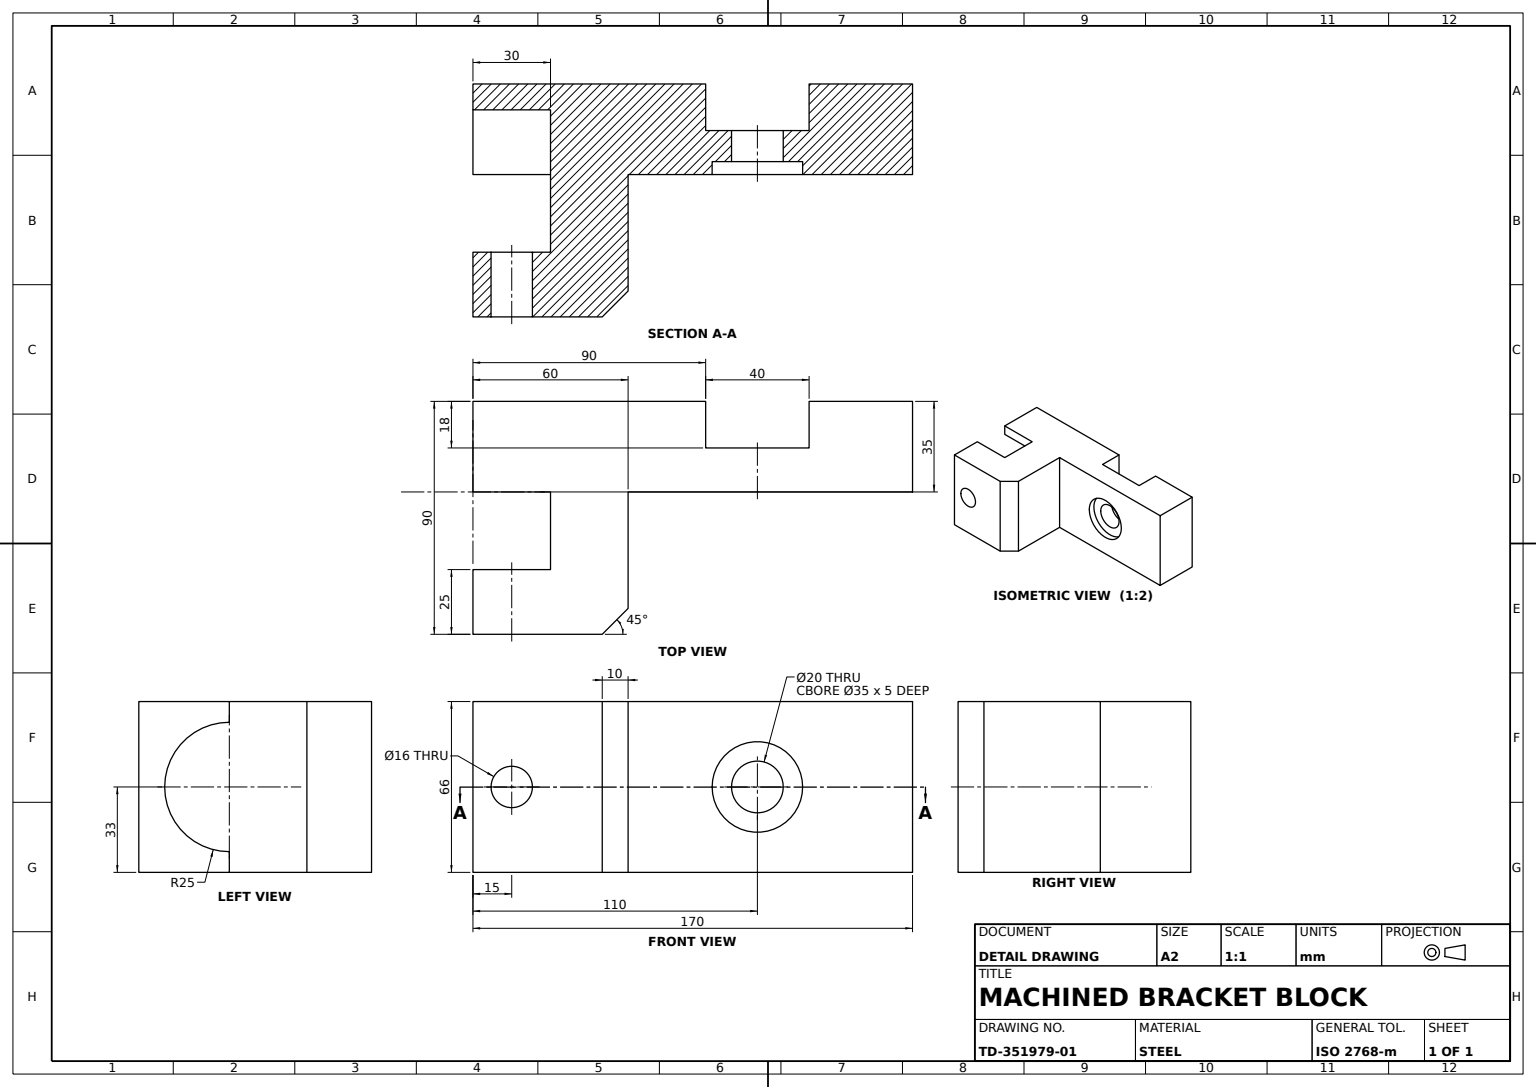
SolidWorks part; units mm, degrees
material "Plain Carbon Steel"
ref_plane "Front Plane" through (0, 0, 0) normal (0, 0, 1) x (1, 0, 0)
ref_plane "Top Plane" through (0, 0, 0) normal (0, 1, 0) x (1, 0, 0)
ref_plane "Right Plane" through (0, 0, 0) normal (1, 0, 0) x (0, 0, -1)
sketch "Base Block Profile" plane through (0, 0, 0) normal (0, 0, 1) x (1, 0, 0)
  line L0 (0, 0) -> (170, 0)
  line L1 (170, 0) -> (170, 66)
  line L2 (170, 66) -> (0, 66)
  line L3 (0, 66) -> (0, 0)
  dimension "D1" = 170
  dimension "D2" = 66
extrude "Base Block" add sketch "Base Block Profile" along normal blind 35
sketch "Slot Profile" plane through (0, 0, 0) normal (0, -1, 0) x (1, 0, 0)
  line L0 (170, 0) -> (110, 0)
  line L1 (0, 0) -> (170, 0) construction
  line L2 (170, 35) -> (170, 0) construction
  line L4 (110, 0) -> (130, 0)
  line L5 (130, 0) -> (90, 0)
  line L6 (130, 0) -> (130, 18)
  line L7 (130, 18) -> (90, 18)
  line L8 (90, 18) -> (90, 0)
  line M1 (0, 0) -> (170, 0)
  dimension "D1" = 40
  dimension "D2" = 60
  dimension "D3" = 18
extrude "Slot Cut" cut sketch "Slot Profile" against normal blind 66 contours L7 L8 L6 M1
sketch "Counterbore Ø35 Sketch" plane through (0, 0, 35) normal (0, 0, 1) x (1, 0, 0)
  line L0 (0, 66) -> (0, 0) construction
  line L1 (0, 0) -> (170, 0) construction
  circle A0 centre (110, 33) radius 17.5
  dimension "D1" = 35
  dimension "D2" = 35
  dimension "D3" = 110
  dimension "D4" = 33
extrude "Counterbore Ø35" cut sketch "Counterbore Ø35 Sketch" against normal blind 5
sketch "Hole Ø20 Sketch" plane through (0, 0, 30) normal (0, 0, 1) x (1, 0, 0)
  circle A0 centre (110, 33) radius 10
  dimension "D1" = 20
  dimension "D2" = 20
extrude "Hole Ø20" cut sketch "Hole Ø20 Sketch" against normal blind 12
sketch "Rounded Cut Sketch" plane through (0, 0, 0) normal (-1, 0, 0) x (0, 0, 1)
  line L0 (35, 66) -> (35, 0) construction
  line L1 (35, 58) -> (35, 8)
  arc A0 (35, 58) -> (35, 8) centre (35, 33) ccw
  dimension "D1" = 50
  dimension "D2" = 25
extrude "Rounded Cut" cut sketch "Rounded Cut Sketch" against normal blind 30
sketch "Side Lug Profile" plane through (0, 0, 0) normal (0, -1, 0) x (1, 0, 0)
  line L0 (170, 35) -> (170, 0) construction
  line L1 (0, 35) -> (170, 35) construction
  line L2 (30, 35) -> (30, 65)
  line L3 (30, 65) -> (0, 65)
  line L4 (0, 65) -> (0, 90)
  line L5 (0, 90) -> (50, 90)
  line L8 (60, 80) -> (60, 35)
  line L9 (60, 35) -> (30, 35)
  line L10 (50, 90) -> (60, 80)
  line L11 (30, 35) -> (60, 35)
  line L12 (130, 18) -> (90, 18) construction
  line M5 (170, 35) -> (0, 35)
  dimension "D1" = 110
  dimension "D2" = 120
  dimension "D3" = 62
  dimension "D4" = 72
extrude "Side Lug" add sketch "Side Lug Profile" against normal blind 66 contours L10 L5 L4 L3 L2 L8 M5
sketch "Lug Hole Ø16 Sketch" plane through (0, 0, 90) normal (0, 0, 1) x (1, 0, 0)
  line L0 (0, 66) -> (0, 0) construction
  line L2 (0, 0) -> (50, 0) construction
  circle A0 centre (15, 33) radius 8
  dimension "D1" = 16
  dimension "D3" = 16
  dimension "D2" = 15
  dimension "D4" = 33
extrude "Lug Hole Ø16" cut sketch "Lug Hole Ø16 Sketch" against normal blind 66
